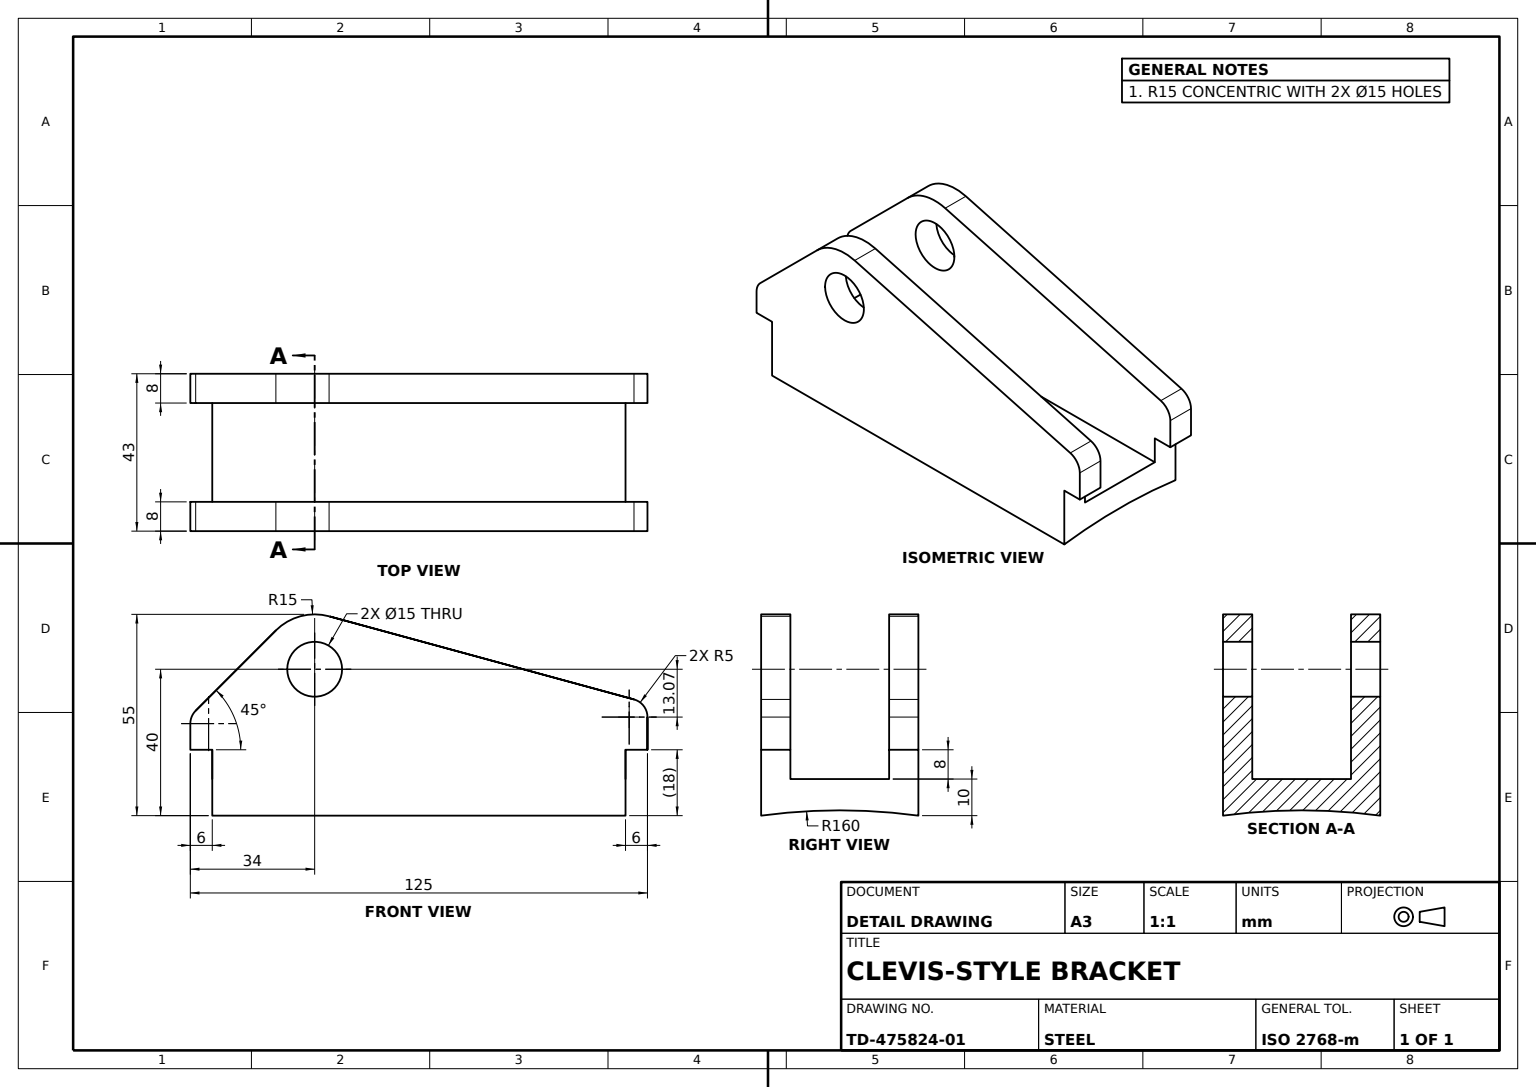
from build123d import *

# Parameters (mm, degrees)
CLEVIS_PROFILE_SKETCH_R = 7.5
CLEVIS_BODY_DEPTH       = 21.5
CLEVIS_GAP_SKETCH_W     = 27
CLEVIS_GAP_SKETCH_H     = 45
CLEVIS_GAP_CUT_DEPTH    = 186.5


with BuildPart() as part:
    # Clevis Profile Sketch → Clevis Body (new, symmetric)
    with BuildSketch(Plane.XY):
        with BuildLine():
            ThreePointArc((-34, -14.857864376), (-33.619397663, -12.944447214), (-32.535533906, -11.32233047))
            Line((-32.535533906, -11.32233047), (-10.606601718, 10.606601718))
            ThreePointArc((-10.606601718, 10.606601718), (-3.851711358, 14.497045203), (3.943382345, 14.47237837))
            Line((3.943382345, 14.47237837), (87.314460782, -8.24427748))
            ThreePointArc((87.314460782, -8.24427748), (89.973179074, -10.032971502), (91, -13.068403604))
            Line((91, -13.068403604), (91, -22))
            Line((91, -22), (85, -22))
            Line((85, -22), (85, -40))
            Line((85, -40), (-28, -40))
            Line((-28, -40), (-28, -22))
            Line((-28, -22), (-34, -22))
            Line((-34, -22), (-34, -14.857864376))
        make_face()
        Circle(CLEVIS_PROFILE_SKETCH_R, mode=Mode.SUBTRACT)
    extrude(amount=CLEVIS_BODY_DEPTH, both=True)

    # Clevis Gap Sketch → Clevis Gap Cut (cut, symmetric)
    with BuildSketch(Plane(origin=(85, 0, 0), x_dir=(0, 0, -1), z_dir=(1, 0, 0))):
        with Locations((0, -7.5)):
            Rectangle(CLEVIS_GAP_SKETCH_W, CLEVIS_GAP_SKETCH_H)
        with BuildLine():
            Line((-21.5, -40), (21.5, -40))
            ThreePointArc((21.5, -40), (0, -38.548888359), (-21.5, -40))
        make_face()
    extrude(amount=CLEVIS_GAP_CUT_DEPTH, both=True, mode=Mode.SUBTRACT)


solid = part.part
